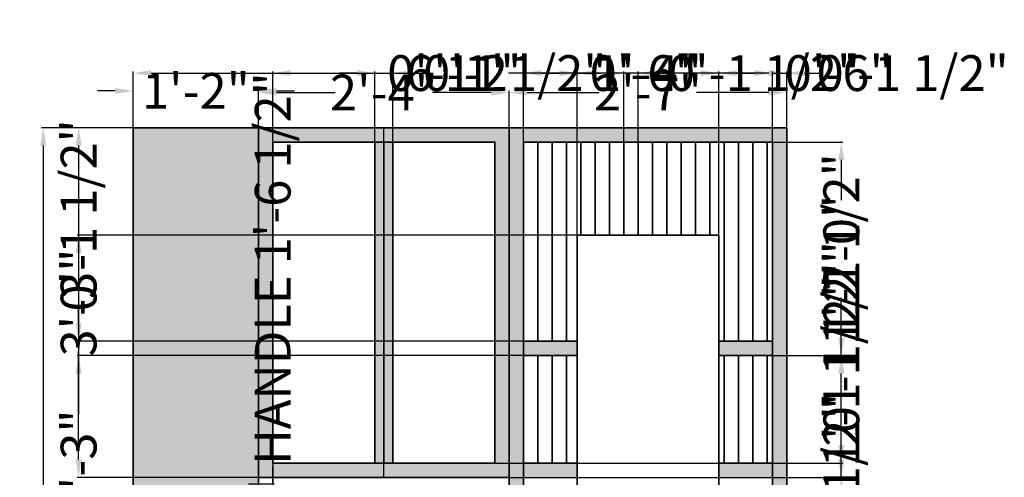
# Model space of a CAD drawing. Units: inches. Extents: x 15 to 125, y 28 to 155.
# Tile 2 of 2: x 15 to 125, y 104 to 155. Entities that reach past the tile are written whole.
import ezdxf

# ---------------------------------------------------------------- set-up
doc = ezdxf.new("R2010")
doc.units = ezdxf.units.IN
doc.header["$MEASUREMENT"] = 0
for name, color, linetype, lineweight in [('A-ANNO-DIMS', 2, 'Continuous', 18), ('A-FURN', 7, 'Continuous', 35), ('A-FURN-PATT', 252, 'Continuous', 13), ('A-GLAZ', 4, 'Continuous', 25)]:
    doc.layers.add(name, color=color, linetype=linetype, lineweight=lineweight)
doc.styles.get("Standard").update_dxf_attribs({"font": 'arial.ttf'})
doc.dimstyles.get("Standard").update_dxf_attribs({"dimtxt": 4, "dimasz": 2, "dimexe": 0.18, "dimexo": 0.0625, "dimgap": 0.09, "dimtad": 0, "dimdec": 0, "dimzin": 0, "dimdsep": 46, "dimlunit": 4, "dimtxsty": 'Standard', "dimcen": 0.09, "dimadec": 0, "dimazin": 0, "dimtfac": 1, "dimtdec": 0, "dimtofl": 0, "dimtmove": 0, "dimatfit": 3, "dimfxl": 1, "dimtolj": 1, "dimtzin": 0, "dimarcsym": 0})

# ---------------------------------------------------------------- blocks, each defined once
blk = doc.blocks.new('*D5')
at = {"layer": 'A-ANNO-DIMS', "color": 0, "lineweight": -2, "transparency": 16777216}
for p, q in [((69.43, 142.93), (69.43, 146.98)), ((71.43, 146.8), (79.49, 146.8)), ((98.43, 146.8), (90.37, 146.8)), ((100.43, 142.93), (100.43, 146.98))]:
    blk.add_line(p, q, dxfattribs=at)
at = {"layer": 'A-ANNO-DIMS', "color": 0, "transparency": 16777216}
for points in [[(71.43, 147.13), (71.43, 146.47), (69.43, 146.8)], [(98.43, 147.13), (98.43, 146.47), (100.43, 146.8)]]:
    blk.add_solid(points, dxfattribs=at)
at = {"layer": 'Defpoints', "color": 0, "transparency": 16777216}
for p in [(100.43, 146.8), (69.43, 142.87), (100.43, 142.87)]:
    blk.add_point(p, dxfattribs=at)
at = {"layer": 'A-ANNO-DIMS', "color": 0, "transparency": 16777216, "insert": (84.93, 146.8), "char_height": 4, "attachment_point": 5}
blk.add_mtext('\\A1;2\'-7"', dxfattribs=at)
blk = doc.blocks.new('*D6')
at = {"layer": 'A-ANNO-DIMS', "color": 0, "lineweight": -2, "transparency": 16777216}
for p, q in [((41.43, 142.93), (41.43, 146.98)), ((43.43, 146.8), (49.99, 146.8)), ((67.43, 146.8), (60.87, 146.8)), ((69.43, 142.93), (69.43, 146.98))]:
    blk.add_line(p, q, dxfattribs=at)
at = {"layer": 'A-ANNO-DIMS', "color": 0, "transparency": 16777216}
for points in [[(43.43, 147.13), (43.43, 146.47), (41.43, 146.8)], [(67.43, 147.13), (67.43, 146.47), (69.43, 146.8)]]:
    blk.add_solid(points, dxfattribs=at)
at = {"layer": 'Defpoints', "color": 0, "transparency": 16777216}
for p in [(69.43, 146.8), (41.43, 142.87), (69.43, 142.87)]:
    blk.add_point(p, dxfattribs=at)
at = {"layer": 'A-ANNO-DIMS', "color": 0, "transparency": 16777216, "insert": (55.43, 146.8), "char_height": 4, "attachment_point": 5}
blk.add_mtext('\\A1;2\'-4"', dxfattribs=at)
blk = doc.blocks.new('*D7')
at = {"layer": 'A-ANNO-DIMS', "color": 0, "lineweight": -2, "transparency": 16777216}
for p, q in [((25.43, 146.98), (23.43, 146.98)), ((27.43, 142.93), (27.43, 147.16)), ((41.43, 142.93), (41.43, 147.16)), ((43.43, 146.98), (45.43, 146.98))]:
    blk.add_line(p, q, dxfattribs=at)
at = {"layer": 'A-ANNO-DIMS', "color": 0, "transparency": 16777216}
for points in [[(25.43, 147.31), (25.43, 146.65), (27.43, 146.98)], [(43.43, 147.31), (43.43, 146.65), (41.43, 146.98)]]:
    blk.add_solid(points, dxfattribs=at)
at = {"layer": 'Defpoints', "color": 0, "transparency": 16777216}
for p in [(41.43, 146.98), (27.43, 142.87), (41.43, 142.87)]:
    blk.add_point(p, dxfattribs=at)
at = {"layer": 'A-ANNO-DIMS', "color": 0, "transparency": 16777216, "insert": (34.43, 146.98), "char_height": 4, "attachment_point": 5}
blk.add_mtext('\\A1;1\'-2"', dxfattribs=at)
blk = doc.blocks.new('*D8')
at = {"layer": 'A-ANNO-DIMS', "color": 0, "lineweight": -2, "transparency": 16777216}
for p, q in [((27.37, 142.87), (17.19, 142.87)), ((17.37, 140.87), (17.37, 102.26)), ((17.37, 52.87), (17.37, 91.48)), ((27.37, 50.87), (17.19, 50.87))]:
    blk.add_line(p, q, dxfattribs=at)
at = {"layer": 'A-ANNO-DIMS', "color": 0, "transparency": 16777216}
for points in [[(17.04, 140.87), (17.7, 140.87), (17.37, 142.87)], [(17.04, 52.87), (17.7, 52.87), (17.37, 50.87)]]:
    blk.add_solid(points, dxfattribs=at)
at = {"layer": 'Defpoints', "color": 0, "transparency": 16777216}
for p in [(27.43, 142.87), (17.37, 50.87), (27.43, 50.87)]:
    blk.add_point(p, dxfattribs=at)
at = {"layer": 'A-ANNO-DIMS', "color": 0, "transparency": 16777216, "insert": (17.37, 96.87), "char_height": 4, "attachment_point": 5, "rotation": 90}
blk.add_mtext('\\A1;7\'-8"', dxfattribs=at)
blk = doc.blocks.new('*D11')
at = {"layer": 'A-ANNO-DIMS', "color": 0, "lineweight": -2, "transparency": 16777216}
for p, q in [((43.01, 103.07), (43.01, 105.07)), ((40.31, 103.07), (43.19, 103.07)), ((43.01, 86.71), (43.01, 101.07)), ((40.31, 84.71), (43.19, 84.71))]:
    blk.add_line(p, q, dxfattribs=at)
at = {"layer": 'A-ANNO-DIMS', "color": 0, "transparency": 16777216}
for points in [[(42.67, 101.07), (43.34, 101.07), (43.01, 103.07)], [(42.67, 86.71), (43.34, 86.71), (43.01, 84.71)]]:
    blk.add_solid(points, dxfattribs=at)
at = {"layer": 'Defpoints', "color": 0, "transparency": 16777216}
for p in [(40.25, 103.07), (43.01, 103.07), (40.25, 84.71)]:
    blk.add_point(p, dxfattribs=at)
at = {"layer": 'A-ANNO-DIMS', "color": 0, "transparency": 16777216, "insert": (43.01, 127.14), "char_height": 4, "attachment_point": 5, "rotation": 90}
blk.add_mtext('\\A1;HANDLE 1\'-6 1/2"', dxfattribs=at)
blk = doc.blocks.new('*D13')
at = {"layer": 'A-ANNO-DIMS', "color": 0, "lineweight": -2, "transparency": 16777216}
for p, q in [((27.43, 142.93), (27.43, 149.15)), ((29.43, 148.97), (58.51, 148.97)), ((98.43, 148.97), (69.35, 148.97)), ((100.43, 142.93), (100.43, 149.15))]:
    blk.add_line(p, q, dxfattribs=at)
at = {"layer": 'A-ANNO-DIMS', "color": 0, "transparency": 16777216}
for points in [[(29.43, 149.3), (29.43, 148.64), (27.43, 148.97)], [(98.43, 149.3), (98.43, 148.64), (100.43, 148.97)]]:
    blk.add_solid(points, dxfattribs=at)
at = {"layer": 'Defpoints', "color": 0, "transparency": 16777216}
for p in [(100.43, 148.97), (27.43, 142.87), (100.43, 142.87)]:
    blk.add_point(p, dxfattribs=at)
at = {"layer": 'A-ANNO-DIMS', "color": 0, "transparency": 16777216, "insert": (63.93, 148.97), "char_height": 4, "attachment_point": 5}
blk.add_mtext('\\A1;6\'-1"', dxfattribs=at)
blk = doc.blocks.new('*D14')
at = {"layer": 'A-ANNO-DIMS', "color": 0, "lineweight": -2, "transparency": 16777216}
for p, q in [((41.43, 142.81), (41.43, 44.59)), ((69.43, 50.81), (69.43, 44.59)), ((43.43, 44.77), (49.99, 44.77)), ((67.43, 44.77), (60.87, 44.77))]:
    blk.add_line(p, q, dxfattribs=at)
at = {"layer": 'A-ANNO-DIMS', "color": 0, "transparency": 16777216}
for points in [[(43.43, 45.1), (43.43, 44.44), (41.43, 44.77)], [(67.43, 45.1), (67.43, 44.44), (69.43, 44.77)]]:
    blk.add_solid(points, dxfattribs=at)
at = {"layer": 'Defpoints', "color": 0, "transparency": 16777216}
for p in [(41.43, 142.87), (69.43, 50.87), (69.43, 44.77)]:
    blk.add_point(p, dxfattribs=at)
at = {"layer": 'A-ANNO-DIMS', "color": 0, "transparency": 16777216, "insert": (55.43, 44.77), "char_height": 4, "attachment_point": 5}
blk.add_mtext('\\A1;2\'-4"', dxfattribs=at)
blk = doc.blocks.new('*D18')
at = {"layer": 'A-ANNO-DIMS', "color": 0, "lineweight": -2, "transparency": 16777216}
for p, q in [((43.03, 105.35), (43.03, 44.59)), ((41.43, 103.75), (41.43, 44.59)), ((39.43, 44.77), (37.43, 44.77)), ((45.03, 44.77), (47.03, 44.77))]:
    blk.add_line(p, q, dxfattribs=at)
at = {"layer": 'A-ANNO-DIMS', "color": 0, "transparency": 16777216}
for points in [[(39.43, 45.1), (39.43, 44.44), (41.43, 44.77)], [(45.03, 45.1), (45.03, 44.44), (43.03, 44.77)]]:
    blk.add_solid(points, dxfattribs=at)
at = {"layer": 'Defpoints', "color": 0, "transparency": 16777216}
for p in [(43.03, 105.41), (41.43, 103.81), (43.03, 44.77)]:
    blk.add_point(p, dxfattribs=at)
at = {"layer": 'A-ANNO-DIMS', "color": 0, "transparency": 16777216, "insert": (57.1, 44.77), "char_height": 4, "attachment_point": 5}
blk.add_mtext('\\A1;0\'-1 1/2"', dxfattribs=at)
blk = doc.blocks.new('*D19')
at = {"layer": 'A-ANNO-DIMS', "color": 0, "lineweight": -2, "transparency": 16777216}
for p, q in [((43.03, 141.33), (43.03, 149.15)), ((45.03, 148.97), (52.43, 148.97)), ((54.43, 141.33), (54.43, 149.15)), ((54.43, 148.97), (56.43, 148.97))]:
    blk.add_line(p, q, dxfattribs=at)
at = {"layer": 'A-ANNO-DIMS', "color": 0, "transparency": 16777216}
for points in [[(45.03, 149.3), (45.03, 148.64), (43.03, 148.97)], [(52.43, 149.3), (52.43, 148.64), (54.43, 148.97)]]:
    blk.add_solid(points, dxfattribs=at)
at = {"layer": 'Defpoints', "color": 0, "transparency": 16777216}
for p in [(54.43, 148.97), (43.03, 141.27), (54.43, 141.27)]:
    blk.add_point(p, dxfattribs=at)
at = {"layer": 'A-ANNO-DIMS', "color": 0, "transparency": 16777216, "insert": (68.05, 148.97), "char_height": 4, "attachment_point": 5}
blk.add_mtext('\\A1;0\'-11 1/2"', dxfattribs=at)
blk = doc.blocks.new('*D20')
at = {"layer": 'A-ANNO-DIMS', "color": 0, "lineweight": -2, "transparency": 16777216}
for p, q in [((52.43, 148.97), (50.43, 148.97)), ((54.43, 141.33), (54.43, 149.15)), ((56.43, 141.33), (56.43, 149.15)), ((58.43, 148.97), (60.43, 148.97))]:
    blk.add_line(p, q, dxfattribs=at)
at = {"layer": 'A-ANNO-DIMS', "color": 0, "transparency": 16777216}
for points in [[(52.43, 149.3), (52.43, 148.64), (54.43, 148.97)], [(58.43, 149.3), (58.43, 148.64), (56.43, 148.97)]]:
    blk.add_solid(points, dxfattribs=at)
at = {"layer": 'Defpoints', "color": 0, "transparency": 16777216}
for p in [(56.43, 148.97), (54.43, 141.27), (56.43, 141.27)]:
    blk.add_point(p, dxfattribs=at)
at = {"layer": 'A-ANNO-DIMS', "color": 0, "transparency": 16777216, "insert": (65.84, 148.97), "char_height": 4, "attachment_point": 5}
blk.add_mtext('\\A1;0\'-2"', dxfattribs=at)
blk = doc.blocks.new('*D21')
at = {"layer": 'A-ANNO-DIMS', "color": 0, "lineweight": -2, "transparency": 16777216}
for p, q in [((106.53, 107.41), (106.53, 109.41)), ((56.49, 105.41), (106.71, 105.41)), ((55.49, 103.81), (106.71, 103.81)), ((106.53, 101.81), (106.53, 99.81))]:
    blk.add_line(p, q, dxfattribs=at)
at = {"layer": 'A-ANNO-DIMS', "color": 0, "transparency": 16777216}
for points in [[(106.2, 107.41), (106.86, 107.41), (106.53, 105.41)], [(106.2, 101.81), (106.86, 101.81), (106.53, 103.81)]]:
    blk.add_solid(points, dxfattribs=at)
at = {"layer": 'Defpoints', "color": 0, "transparency": 16777216}
for p in [(56.43, 105.41), (106.53, 105.41), (55.43, 103.81)]:
    blk.add_point(p, dxfattribs=at)
at = {"layer": 'A-ANNO-DIMS', "color": 0, "transparency": 16777216, "insert": (106.53, 119.48), "char_height": 4, "attachment_point": 5, "rotation": 90}
blk.add_mtext('\\A1;0\'-1 1/2"', dxfattribs=at)
blk = doc.blocks.new('*D22')
at = {"layer": 'A-ANNO-DIMS', "color": 0, "lineweight": -2, "transparency": 16777216}
for p, q in [((41.37, 142.87), (21.15, 142.87)), ((21.33, 140.87), (21.33, 128.75)), ((21.33, 105.81), (21.33, 117.94)), ((41.37, 103.81), (21.15, 103.81))]:
    blk.add_line(p, q, dxfattribs=at)
at = {"layer": 'A-ANNO-DIMS', "color": 0, "transparency": 16777216}
for points in [[(21, 140.87), (21.66, 140.87), (21.33, 142.87)], [(21, 105.81), (21.66, 105.81), (21.33, 103.81)]]:
    blk.add_solid(points, dxfattribs=at)
at = {"layer": 'Defpoints', "color": 0, "transparency": 16777216}
for p in [(21.33, 142.87), (41.43, 142.87), (41.43, 103.81)]:
    blk.add_point(p, dxfattribs=at)
at = {"layer": 'A-ANNO-DIMS', "color": 0, "transparency": 16777216, "insert": (21.33, 123.34), "char_height": 4, "attachment_point": 5, "rotation": 90}
blk.add_mtext('\\A1;3\'-3"', dxfattribs=at)
blk = doc.blocks.new('*D29')
at = {"layer": 'A-ANNO-DIMS', "color": 0, "lineweight": -2, "transparency": 16777216}
for p, q in [((96.83, 148.97), (94.83, 148.97)), ((98.83, 74.93), (98.83, 149.15)), ((100.43, 50.93), (100.43, 149.15)), ((102.43, 148.97), (104.43, 148.97))]:
    blk.add_line(p, q, dxfattribs=at)
at = {"layer": 'A-ANNO-DIMS', "color": 0, "transparency": 16777216}
for points in [[(96.83, 149.3), (96.83, 148.64), (98.83, 148.97)], [(102.43, 149.3), (102.43, 148.64), (100.43, 148.97)]]:
    blk.add_solid(points, dxfattribs=at)
at = {"layer": 'Defpoints', "color": 0, "transparency": 16777216}
for p in [(100.43, 148.97), (98.83, 74.87), (100.43, 50.87)]:
    blk.add_point(p, dxfattribs=at)
at = {"layer": 'A-ANNO-DIMS', "color": 0, "transparency": 16777216, "insert": (114.5, 148.97), "char_height": 4, "attachment_point": 5}
blk.add_mtext('\\A1;0\'-1 1/2"', dxfattribs=at)
blk = doc.blocks.new('*D30')
at = {"layer": 'A-ANNO-DIMS', "color": 0, "lineweight": -2, "transparency": 16777216}
for p, q in [((80.23, 148.97), (78.23, 148.97)), ((82.23, 141.33), (82.23, 149.15)), ((83.83, 141.33), (83.83, 149.15)), ((85.83, 148.97), (87.83, 148.97))]:
    blk.add_line(p, q, dxfattribs=at)
at = {"layer": 'A-ANNO-DIMS', "color": 0, "transparency": 16777216}
for points in [[(80.23, 149.3), (80.23, 148.64), (82.23, 148.97)], [(85.83, 149.3), (85.83, 148.64), (83.83, 148.97)]]:
    blk.add_solid(points, dxfattribs=at)
at = {"layer": 'Defpoints', "color": 0, "transparency": 16777216}
for p in [(83.83, 148.97), (82.23, 141.27), (83.83, 141.27)]:
    blk.add_point(p, dxfattribs=at)
at = {"layer": 'A-ANNO-DIMS', "color": 0, "transparency": 16777216, "insert": (97.9, 148.97), "char_height": 4, "attachment_point": 5}
blk.add_mtext('\\A1;0\'-1 1/2"', dxfattribs=at)
blk = doc.blocks.new('*D31')
at = {"layer": 'A-ANNO-DIMS', "color": 0, "lineweight": -2, "transparency": 16777216}
for p, q in [((71.03, 119.08), (71.03, 149.15)), ((73.03, 148.97), (75.03, 148.97)), ((77.03, 119.08), (77.03, 149.15)), ((77.03, 148.97), (79.03, 148.97))]:
    blk.add_line(p, q, dxfattribs=at)
at = {"layer": 'A-ANNO-DIMS', "color": 0, "transparency": 16777216}
for points in [[(73.03, 149.3), (73.03, 148.64), (71.03, 148.97)], [(75.03, 149.3), (75.03, 148.64), (77.03, 148.97)]]:
    blk.add_solid(points, dxfattribs=at)
at = {"layer": 'Defpoints', "color": 0, "transparency": 16777216}
for p in [(77.03, 148.97), (71.03, 119.01), (77.03, 119.01)]:
    blk.add_point(p, dxfattribs=at)
at = {"layer": 'A-ANNO-DIMS', "color": 0, "transparency": 16777216, "insert": (84.44, 148.97), "char_height": 4, "attachment_point": 5}
blk.add_mtext('\\A1;0\'-6"', dxfattribs=at)
blk = doc.blocks.new('*D32')
at = {"layer": 'A-ANNO-DIMS', "color": 0, "lineweight": -2, "transparency": 16777216}
for p, q in [((77.03, 130.93), (77.03, 149.15)), ((79.03, 148.97), (79.71, 148.97)), ((90.83, 148.97), (90.15, 148.97)), ((92.83, 130.93), (92.83, 149.15))]:
    blk.add_line(p, q, dxfattribs=at)
at = {"layer": 'A-ANNO-DIMS', "color": 0, "transparency": 16777216}
for points in [[(79.03, 149.3), (79.03, 148.64), (77.03, 148.97)], [(90.83, 149.3), (90.83, 148.64), (92.83, 148.97)]]:
    blk.add_solid(points, dxfattribs=at)
at = {"layer": 'Defpoints', "color": 0, "transparency": 16777216}
for p in [(92.83, 148.97), (77.03, 130.87), (92.83, 130.87)]:
    blk.add_point(p, dxfattribs=at)
at = {"layer": 'A-ANNO-DIMS', "color": 0, "transparency": 16777216, "insert": (84.93, 148.97), "char_height": 4, "attachment_point": 5}
blk.add_mtext('\\A1;1\'-4"', dxfattribs=at)
blk = doc.blocks.new('*D33')
at = {"layer": 'A-ANNO-DIMS', "color": 0, "lineweight": -2, "transparency": 16777216}
for p, q in [((76.97, 130.87), (21.15, 130.87)), ((21.33, 128.87), (21.33, 110.86)), ((21.33, 81.87), (21.33, 99.88)), ((76.97, 79.87), (21.15, 79.87))]:
    blk.add_line(p, q, dxfattribs=at)
at = {"layer": 'A-ANNO-DIMS', "color": 0, "transparency": 16777216}
for points in [[(21, 128.87), (21.66, 128.87), (21.33, 130.87)], [(21, 81.87), (21.66, 81.87), (21.33, 79.87)]]:
    blk.add_solid(points, dxfattribs=at)
at = {"layer": 'Defpoints', "color": 0, "transparency": 16777216}
for p in [(21.33, 130.87), (77.03, 130.87), (77.03, 79.87)]:
    blk.add_point(p, dxfattribs=at)
at = {"layer": 'A-ANNO-DIMS', "color": 0, "transparency": 16777216, "insert": (21.33, 105.37), "char_height": 4, "attachment_point": 5, "rotation": 90}
blk.add_mtext('\\A1;4\'-3"', dxfattribs=at)
blk = doc.blocks.new('*D34')
at = {"layer": 'A-ANNO-DIMS', "color": 0, "lineweight": -2, "transparency": 16777216}
for p, q in [((106.53, 90.21), (106.53, 92.21)), ((98.89, 90.21), (106.71, 90.21)), ((106.53, 76.87), (106.53, 88.21)), ((98.89, 74.87), (106.71, 74.87))]:
    blk.add_line(p, q, dxfattribs=at)
at = {"layer": 'A-ANNO-DIMS', "color": 0, "transparency": 16777216}
for points in [[(106.2, 88.21), (106.86, 88.21), (106.53, 90.21)], [(106.2, 76.87), (106.86, 76.87), (106.53, 74.87)]]:
    blk.add_solid(points, dxfattribs=at)
at = {"layer": 'Defpoints', "color": 0, "transparency": 16777216}
for p in [(98.83, 90.21), (106.53, 90.21), (98.83, 74.87)]:
    blk.add_point(p, dxfattribs=at)
at = {"layer": 'A-ANNO-DIMS', "color": 0, "transparency": 16777216, "insert": (106.53, 102.09), "char_height": 4, "attachment_point": 5, "rotation": 90}
blk.add_mtext('\\A1;1\'-3 1/2"', dxfattribs=at)
blk = doc.blocks.new('*D35')
at = {"layer": 'A-ANNO-DIMS', "color": 0, "lineweight": -2, "transparency": 16777216}
for p, q in [((106.53, 103.81), (106.53, 105.81)), ((98.89, 103.81), (106.71, 103.81)), ((106.53, 92.21), (106.53, 101.81)), ((98.89, 90.21), (106.71, 90.21))]:
    blk.add_line(p, q, dxfattribs=at)
at = {"layer": 'A-ANNO-DIMS', "color": 0, "transparency": 16777216}
for points in [[(106.2, 101.81), (106.86, 101.81), (106.53, 103.81)], [(106.2, 92.21), (106.86, 92.21), (106.53, 90.21)]]:
    blk.add_solid(points, dxfattribs=at)
at = {"layer": 'Defpoints', "color": 0, "transparency": 16777216}
for p in [(98.83, 103.81), (106.53, 103.81), (98.83, 90.21)]:
    blk.add_point(p, dxfattribs=at)
at = {"layer": 'A-ANNO-DIMS', "color": 0, "transparency": 16777216, "insert": (106.53, 115.69), "char_height": 4, "attachment_point": 5, "rotation": 90}
blk.add_mtext('\\A1;1\'-1 1/2"', dxfattribs=at)
blk = doc.blocks.new('*D36')
at = {"layer": 'A-ANNO-DIMS', "color": 0, "lineweight": -2, "transparency": 16777216}
for p, q in [((106.53, 117.41), (106.53, 119.41)), ((98.89, 117.41), (106.71, 117.41)), ((106.53, 105.81), (106.53, 115.41)), ((98.89, 103.81), (106.71, 103.81))]:
    blk.add_line(p, q, dxfattribs=at)
at = {"layer": 'A-ANNO-DIMS', "color": 0, "transparency": 16777216}
for points in [[(106.2, 115.41), (106.86, 115.41), (106.53, 117.41)], [(106.2, 105.81), (106.86, 105.81), (106.53, 103.81)]]:
    blk.add_solid(points, dxfattribs=at)
at = {"layer": 'Defpoints', "color": 0, "transparency": 16777216}
for p in [(98.83, 117.41), (106.53, 117.41), (98.83, 103.81)]:
    blk.add_point(p, dxfattribs=at)
at = {"layer": 'A-ANNO-DIMS', "color": 0, "transparency": 16777216, "insert": (106.53, 129.29), "char_height": 4, "attachment_point": 5, "rotation": 90}
blk.add_mtext('\\A1;1\'-1 1/2"', dxfattribs=at)
blk = doc.blocks.new('*D37')
at = {"layer": 'A-ANNO-DIMS', "color": 0, "lineweight": -2, "transparency": 16777216}
for p, q in [((98.89, 141.27), (106.71, 141.27)), ((106.53, 139.27), (106.53, 134.78)), ((106.53, 119.41), (106.53, 123.9)), ((98.89, 117.41), (106.71, 117.41))]:
    blk.add_line(p, q, dxfattribs=at)
at = {"layer": 'A-ANNO-DIMS', "color": 0, "transparency": 16777216}
for points in [[(106.2, 139.27), (106.86, 139.27), (106.53, 141.27)], [(106.2, 119.41), (106.86, 119.41), (106.53, 117.41)]]:
    blk.add_solid(points, dxfattribs=at)
at = {"layer": 'Defpoints', "color": 0, "transparency": 16777216}
for p in [(98.83, 141.27), (106.53, 141.27), (98.83, 117.41)]:
    blk.add_point(p, dxfattribs=at)
at = {"layer": 'A-ANNO-DIMS', "color": 0, "transparency": 16777216, "insert": (106.53, 129.34), "char_height": 4, "attachment_point": 5, "rotation": 90}
blk.add_mtext('\\A1;2\'-0"', dxfattribs=at)
blk = doc.blocks.new('*D38')
at = {"layer": 'A-ANNO-DIMS', "color": 0, "lineweight": -2, "transparency": 16777216}
for p, q in [((21.33, 121.01), (21.33, 123.01)), ((70.97, 119.01), (21.15, 119.01)), ((70.97, 117.41), (21.15, 117.41)), ((21.33, 115.41), (21.33, 113.41))]:
    blk.add_line(p, q, dxfattribs=at)
at = {"layer": 'A-ANNO-DIMS', "color": 0, "transparency": 16777216}
for points in [[(21, 121.01), (21.66, 121.01), (21.33, 119.01)], [(21, 115.41), (21.66, 115.41), (21.33, 117.41)]]:
    blk.add_solid(points, dxfattribs=at)
at = {"layer": 'Defpoints', "color": 0, "transparency": 16777216}
for p in [(21.33, 119.01), (71.03, 119.01), (71.03, 117.41)]:
    blk.add_point(p, dxfattribs=at)
at = {"layer": 'A-ANNO-DIMS', "color": 0, "transparency": 16777216, "insert": (21.33, 133.08), "char_height": 4, "attachment_point": 5, "rotation": 90}
blk.add_mtext('\\A1;0\'-1 1/2"', dxfattribs=at)
blk = doc.blocks.new('*D44')
at = {"layer": 'A-ANNO-DIMS', "color": 0, "lineweight": -2, "transparency": 16777216}
for p, q in [((92.83, 130.93), (92.83, 149.15)), ((94.83, 148.97), (96.83, 148.97)), ((98.83, 117.48), (98.83, 149.15)), ((98.83, 148.97), (100.83, 148.97))]:
    blk.add_line(p, q, dxfattribs=at)
at = {"layer": 'A-ANNO-DIMS', "color": 0, "transparency": 16777216}
for points in [[(94.83, 149.3), (94.83, 148.64), (92.83, 148.97)], [(96.83, 149.3), (96.83, 148.64), (98.83, 148.97)]]:
    blk.add_solid(points, dxfattribs=at)
at = {"layer": 'Defpoints', "color": 0, "transparency": 16777216}
for p in [(98.83, 148.97), (92.83, 130.87), (98.83, 117.41)]:
    blk.add_point(p, dxfattribs=at)
at = {"layer": 'A-ANNO-DIMS', "color": 0, "transparency": 16777216, "insert": (106.24, 148.97), "char_height": 4, "attachment_point": 5}
blk.add_mtext('\\A1;0\'-6"', dxfattribs=at)

msp = doc.modelspace()

# ---------------------------------------------------------------- hatches: boundary and pattern name
at = {"layer": 'A-FURN-PATT'}
h = msp.add_hatch(color=256, dxfattribs=at)
h.dxf.hatch_style = 1
h.paths.add_polyline_path([(55.43, 80.87), (41.43, 80.87), (41.43, 54.87), (55.43, 54.87)])
h.paths.add_polyline_path([(69.43, 80.87), (55.43, 80.87), (55.43, 54.87), (69.43, 54.87)])
h.paths.add_polyline_path([(41.43, 80.87), (41.43, 142.87), (27.43, 142.87), (27.43, 54.87), (41.43, 54.87)])
h = msp.add_hatch(color=256, dxfattribs=at)
h.dxf.hatch_style = 1
h.paths.add_polyline_path([(41.43, 142.87), (41.43, 103.81), (69.43, 103.81), (69.43, 142.87)])
h.paths.add_polyline_path([(43.03, 141.27), (67.83, 141.27), (67.83, 105.41), (43.03, 105.41)], flags=16)
h.paths.add_polyline_path([(56.43, 141.27), (55.43, 141.27), (55.43, 105.41), (56.43, 105.41)], flags=0)
h.paths.add_polyline_path([(55.43, 141.27), (54.43, 141.27), (54.43, 105.41), (55.43, 105.41)], flags=0)
h = msp.add_hatch(color=256, dxfattribs=at)
h.dxf.hatch_style = 1
h.paths.add_polyline_path([(71.03, 141.27), (98.83, 141.27), (98.83, 50.87), (100.43, 50.87), (100.43, 142.87), (69.43, 142.87), (69.43, 50.87), (71.03, 50.87)])
h = msp.add_hatch(color=256, dxfattribs=at)
h.dxf.hatch_style = 1
h.paths.add_polyline_path([(55.43, 141.27), (54.43, 141.27), (54.43, 105.41), (55.43, 105.41)])
h.paths.add_polyline_path([(56.43, 141.27), (55.43, 141.27), (55.43, 105.41), (56.43, 105.41)])
h = msp.add_hatch(color=256, dxfattribs=at)
h.dxf.hatch_style = 1
h.paths.add_polyline_path([(77.03, 119.01), (71.03, 119.01), (71.03, 117.41), (77.03, 117.41)])
h.paths.add_polyline_path([(98.83, 119.01), (92.83, 119.01), (92.83, 117.41), (98.83, 117.41)])
h.paths.add_polyline_path([(98.83, 105.41), (92.83, 105.41), (92.83, 103.81), (98.83, 103.81)])
h.paths.add_polyline_path([(77.03, 105.41), (71.03, 105.41), (71.03, 103.81), (77.03, 103.81)])
h.paths.add_polyline_path([(98.83, 91.81), (92.83, 91.81), (92.83, 90.21), (98.83, 90.21)])
h.paths.add_polyline_path([(77.03, 91.81), (71.03, 91.81), (71.03, 90.21), (77.03, 90.21)])

# ---------------------------------------------------------------- linework, layer by layer
at = {"layer": 'A-FURN'}
for p, q in [((27.43, 142.87), (41.43, 142.87)), ((27.43, 142.87), (27.43, 50.87)), ((41.43, 142.87), (69.43, 142.87)), ((41.43, 142.87), (41.43, 54.87)), ((54.43, 141.27), (54.43, 105.41)), ((55.43, 141.27), (55.43, 105.41)), ((56.43, 141.27), (56.43, 105.41)), ((72.63, 119.01), (72.63, 141.27)), ((74.23, 119.01), (74.23, 141.27)), ((75.83, 119.01), (75.83, 141.27)), ((77.43, 130.87), (77.43, 141.27)), ((79.03, 130.87), (79.03, 141.27)), ((80.63, 130.87), (80.63, 141.27)), ((82.23, 130.87), (82.23, 141.27)), ((83.83, 130.87), (83.83, 141.27)), ((85.43, 130.87), (85.43, 141.27)), ((87.03, 130.87), (87.03, 141.27)), ((88.63, 130.87), (88.63, 141.27)), ((90.23, 130.87), (90.23, 141.27)), ((91.83, 130.87), (91.83, 141.27)), ((93.43, 119.01), (93.43, 141.27)), ((95.03, 119.01), (95.03, 141.27)), ((96.63, 119.01), (96.63, 141.27)), ((98.23, 119.01), (98.23, 141.27)), ((92.83, 130.87), (77.03, 130.87)), ((77.03, 130.87), (77.03, 80.87)), ((92.83, 130.87), (92.83, 80.87)), ((71.03, 119.01), (77.03, 119.01)), ((92.83, 119.01), (98.83, 119.01)), ((77.03, 117.41), (71.03, 117.41)), ((72.63, 105.41), (72.63, 117.41)), ((74.23, 105.41), (74.23, 117.41)), ((75.83, 105.41), (75.83, 117.41)), ((98.83, 117.41), (92.83, 117.41)), ((93.43, 105.41), (93.43, 117.41)), ((95.03, 105.41), (95.03, 117.41)), ((96.63, 105.41), (96.63, 117.41)), ((98.23, 105.41), (98.23, 117.41)), ((71.03, 105.41), (77.03, 105.41)), ((92.83, 105.41), (98.83, 105.41)), ((69.43, 103.81), (41.43, 103.81))]:
    msp.add_line(p, q, dxfattribs=at)
for points in [[(100.43, 142.87), (100.43, 50.87), (69.43, 50.87), (69.43, 142.87)], [(43.03, 141.27), (67.83, 141.27), (67.83, 105.41), (43.03, 105.41)]]:
    msp.add_lwpolyline(points, close=True, dxfattribs=at)
msp.add_lwpolyline([(98.83, 50.87), (98.83, 141.27), (71.03, 141.27), (71.03, 50.87)], dxfattribs=at)
at = {"layer": 'A-GLAZ'}
for p, q in [((69.43, 142.87), (41.43, 142.87)), ((41.43, 142.87), (41.43, 103.81)), ((55.43, 103.81), (55.43, 142.87)), ((69.43, 103.81), (69.43, 142.87)), ((43.03, 141.27), (54.43, 141.27)), ((43.03, 105.41), (43.03, 141.27)), ((54.43, 141.27), (54.43, 105.41)), ((56.43, 141.27), (67.83, 141.27)), ((56.43, 105.41), (56.43, 141.27)), ((67.83, 141.27), (67.83, 105.41)), ((54.43, 105.41), (43.03, 105.41)), ((67.83, 105.41), (56.43, 105.41)), ((41.43, 103.81), (69.43, 103.81))]:
    msp.add_line(p, q, dxfattribs=at)

# ---------------------------------------------------------------- dimensions: what is measured, and where the dimension line sits
at = {"layer": 'A-ANNO-DIMS'}
for base, p1, p2, override, picture, middle in [((54.43, 148.97), (43.03, 141.27), (54.43, 141.27), {"dimdec": 1, "dimlfac": 1, "dimrnd": 0, "dimzin": 1, "dimdsep": 46, "dimlunit": 4, "dimfrac": 2}, '*D19', (68.05, 148.97)), ((83.83, 148.97), (82.23, 141.27), (83.83, 141.27), {"dimdec": 1, "dimlfac": 1, "dimrnd": 0, "dimzin": 1, "dimdsep": 46, "dimlunit": 4, "dimfrac": 2}, '*D30', (97.9, 148.97)), ((100.43, 148.97), (98.83, 74.87), (100.43, 50.87), {"dimdec": 1, "dimlfac": 1, "dimrnd": 0, "dimzin": 1, "dimdsep": 46, "dimlunit": 4, "dimfrac": 2}, '*D29', (114.5, 148.97)), ((100.43, 148.97), (27.43, 142.87), (100.43, 142.87), {"dimdec": 1, "dimlfac": 1, "dimrnd": 0, "dimzin": 1, "dimdsep": 46, "dimlunit": 4, "dimfrac": 2}, '*D13', (63.93, 148.97)), ((56.43, 148.97), (54.43, 141.27), (56.43, 141.27), {"dimdec": 1, "dimlfac": 1, "dimrnd": 0, "dimzin": 1, "dimdsep": 46, "dimlunit": 4, "dimfrac": 2}, '*D20', (65.84, 148.97)), ((77.03, 148.97), (71.03, 119.01), (77.03, 119.01), {"dimdec": 1, "dimlfac": 1, "dimrnd": 0, "dimzin": 1, "dimdsep": 46, "dimlunit": 4, "dimfrac": 2}, '*D31', (84.44, 148.97)), ((92.83, 148.97), (77.03, 130.87), (92.83, 130.87), {"dimdec": 1, "dimlfac": 1, "dimrnd": 0, "dimzin": 1, "dimdsep": 46, "dimlunit": 4, "dimfrac": 2}, '*D32', (84.93, 148.97)), ((98.83, 148.97), (92.83, 130.87), (98.83, 117.41), {"dimdec": 1, "dimlfac": 1, "dimrnd": 0, "dimzin": 1, "dimdsep": 46, "dimlunit": 4, "dimfrac": 2}, '*D44', (106.24, 148.97)), ((41.43, 146.98), (27.43, 142.87), (41.43, 142.87), {"dimclrd": 0, "dimclre": 0, "dimclrt": 0}, '*D7', (34.43, 146.98)), ((69.43, 146.8), (41.43, 142.87), (69.43, 142.87), {"dimclrd": 0, "dimclre": 0, "dimclrt": 0}, '*D6', (55.43, 146.8)), ((100.43, 146.8), (69.43, 142.87), (100.43, 142.87), {"dimclrd": 0, "dimclre": 0, "dimclrt": 0}, '*D5', (84.93, 146.8)), ((69.43, 44.77), (41.43, 142.87), (69.43, 50.87), {"dimdec": 1, "dimlfac": 1, "dimrnd": 0, "dimzin": 1, "dimdsep": 46, "dimlunit": 4, "dimfrac": 2}, '*D14', (55.43, 44.77)), ((43.03, 44.77), (41.43, 103.81), (43.03, 105.41), {"dimdec": 1, "dimlfac": 1, "dimrnd": 0, "dimzin": 1, "dimdsep": 46, "dimlunit": 4, "dimfrac": 2}, '*D18', (57.1, 44.77))]:
    dim = msp.add_linear_dim(base=base, p1=p1, p2=p2, dimstyle='Standard', override=override, dxfattribs=at)
    dim.commit()
    dim.dimension.update_dxf_attribs({"geometry": picture, "text_midpoint": middle})
dim = msp.add_linear_dim(base=(43.01, 103.07), p1=(40.25, 84.71), p2=(40.25, 103.07), angle=90, text='HANDLE <>', dimstyle='Standard', override={"dimdec": 1, "dimrnd": 0, "dimzin": 1, "dimlunit": 4, "dimfrac": 2}, dxfattribs=at)
dim.commit()
dim.dimension.update_dxf_attribs({"geometry": '*D11', "text_midpoint": (43.01, 127.14)})
for base, p1, p2, override, picture, middle in [((21.33, 119.01), (71.03, 117.41), (71.03, 119.01), {"dimdec": 1, "dimlfac": 1, "dimrnd": 0, "dimzin": 1, "dimdsep": 46, "dimlunit": 4, "dimfrac": 2}, '*D38', (21.33, 133.08)), ((17.37, 50.87), (27.43, 142.87), (27.43, 50.87), {"dimclrd": 0, "dimclre": 0, "dimclrt": 0}, '*D8', (17.37, 96.87)), ((21.33, 142.87), (41.43, 103.81), (41.43, 142.87), {"dimdec": 1, "dimlfac": 1, "dimrnd": 0, "dimzin": 1, "dimdsep": 46, "dimlunit": 4, "dimfrac": 2}, '*D22', (21.33, 123.34)), ((106.53, 141.27), (98.83, 117.41), (98.83, 141.27), {"dimdec": 1, "dimlfac": 1, "dimrnd": 0, "dimzin": 1, "dimdsep": 46, "dimlunit": 4, "dimfrac": 2}, '*D37', (106.53, 129.34)), ((106.53, 117.41), (98.83, 103.81), (98.83, 117.41), {"dimdec": 1, "dimlfac": 1, "dimrnd": 0, "dimzin": 1, "dimdsep": 46, "dimlunit": 4, "dimfrac": 2}, '*D36', (106.53, 129.29)), ((21.33, 130.87), (77.03, 79.87), (77.03, 130.87), {"dimdec": 1, "dimlfac": 1, "dimrnd": 0, "dimzin": 1, "dimdsep": 46, "dimlunit": 4, "dimfrac": 2}, '*D33', (21.33, 105.37)), ((106.53, 105.41), (55.43, 103.81), (56.43, 105.41), {"dimdec": 1, "dimlfac": 1, "dimrnd": 0, "dimzin": 1, "dimdsep": 46, "dimlunit": 4, "dimfrac": 2}, '*D21', (106.53, 119.48)), ((106.53, 103.81), (98.83, 90.21), (98.83, 103.81), {"dimdec": 1, "dimlfac": 1, "dimrnd": 0, "dimzin": 1, "dimdsep": 46, "dimlunit": 4, "dimfrac": 2}, '*D35', (106.53, 115.69)), ((106.53, 90.21), (98.83, 74.87), (98.83, 90.21), {"dimdec": 1, "dimlfac": 1, "dimrnd": 0, "dimzin": 1, "dimdsep": 46, "dimlunit": 4, "dimfrac": 2}, '*D34', (106.53, 102.09))]:
    dim = msp.add_linear_dim(base=base, p1=p1, p2=p2, angle=90, dimstyle='Standard', override=override, dxfattribs=at)
    dim.commit()
    dim.dimension.update_dxf_attribs({"geometry": picture, "text_midpoint": middle})

doc.saveas('drawing.dxf')
